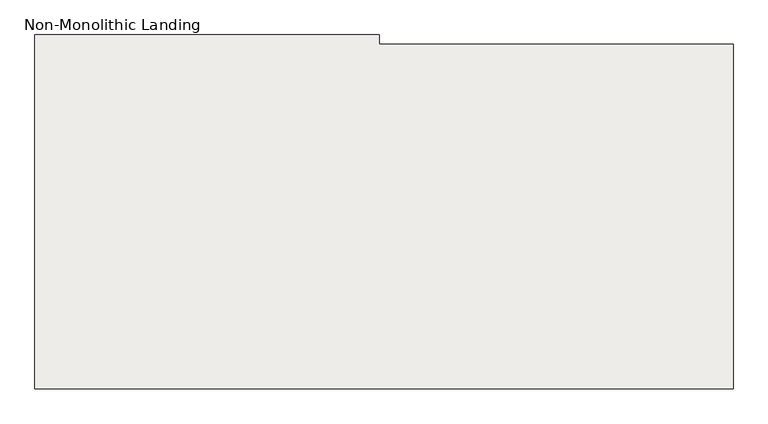
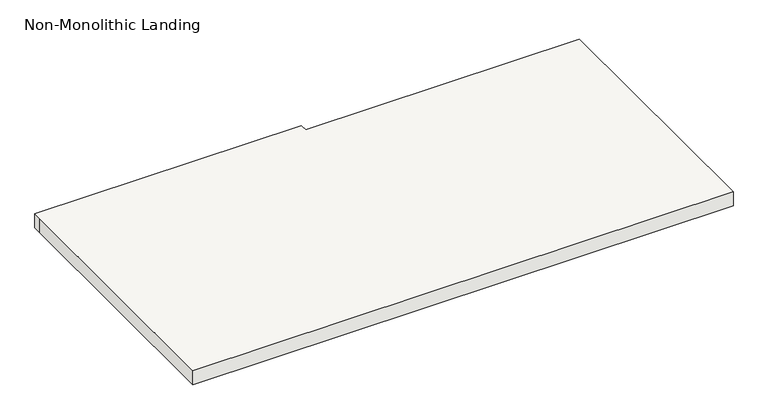
"""IFC4 building model written with IfcOpenShell, lengths in millimetres: slab geometry, Non-Monolithic Landing."""

from ifc_helpers import new_model, si_unit, origin, place, context, project, spatial, faceted_brep, source, transform, mapped, element, save


def non_monolithic_landing_27542c2d(model_context):
    return source(origin(), model_context, "Body", "Brep", [
        faceted_brep([(-2736.9993763, -3538.5064015, 5568.95), (-2736.9993763, -3563.9064015, 5543.55), (-3651.3993763, -3563.9064015, 5543.55), (-3651.3993763, -3538.5064015, 5568.95), (-3676.7993763, -3538.5064015, 5588.0), (-3676.7993763, -3513.1064015, 5588.0), (-4591.1993763, -3513.1064015, 5588.0), (-4591.1993763, -3538.5064015, 5588.0), (-4591.1993763, -4452.9064015, 5588.0), (-2736.9993763, -4452.9064015, 5588.0), (-2736.9993763, -3538.5064015, 5588.0), (-3651.3993763, -3563.9064015, 5537.2), (-2736.9993763, -3563.9064015, 5537.2), (-2736.9993763, -4452.9064015, 5537.2), (-4591.1993763, -4452.9064015, 5537.2), (-4591.1993763, -3538.5064015, 5537.2), (-4591.1993763, -3513.1064015, 5537.2), (-3676.7993763, -3513.1064015, 5537.2), (-3676.7993763, -3538.5064015, 5537.2), (-3651.3993763, -3538.5064015, 5537.2)], [[[0, 1, 2, 3]], [[4, 5, 6, 7, 8, 9, 10]], [[11, 12, 13, 14, 15, 16, 17, 18, 19]], [[12, 11, 2, 1]], [[11, 19, 3, 2]], [[4, 10, 0, 3, 19, 18]], [[5, 4, 18, 17]], [[6, 5, 17, 16]], [[7, 6, 16, 15]], [[8, 7, 15, 14]], [[9, 8, 14, 13]], [[10, 9, 13, 12, 1, 0]]]),
    ])


if __name__ == "__main__":
    model = new_model("IFC4")
    model_context = context("Model", 3, world=origin())
    ifc_project = project(units=[si_unit("LENGTHUNIT", "METRE", prefix="MILLI")], contexts=[model_context])
    site = spatial("IfcSite", under=ifc_project)
    building = spatial("IfcBuilding", under=site)
    placement = place(None, origin())
    non_monolithic_landing_shape = non_monolithic_landing_27542c2d(model_context)
    element("IfcSlab", 1, ObjectType="Non-Monolithic Landing", at=placement, inside=building, context=model_context, shape_type="MappedRepresentation", body=[
        mapped(non_monolithic_landing_shape, transform((0.0, 0.0, 0.0), x_axis=(1.0, 0.0, 0.0), y_axis=(0.0, 1.0, 0.0), z_axis=(0.0, 0.0, 1.0))),
    ])
    save(model, "model.ifc")
